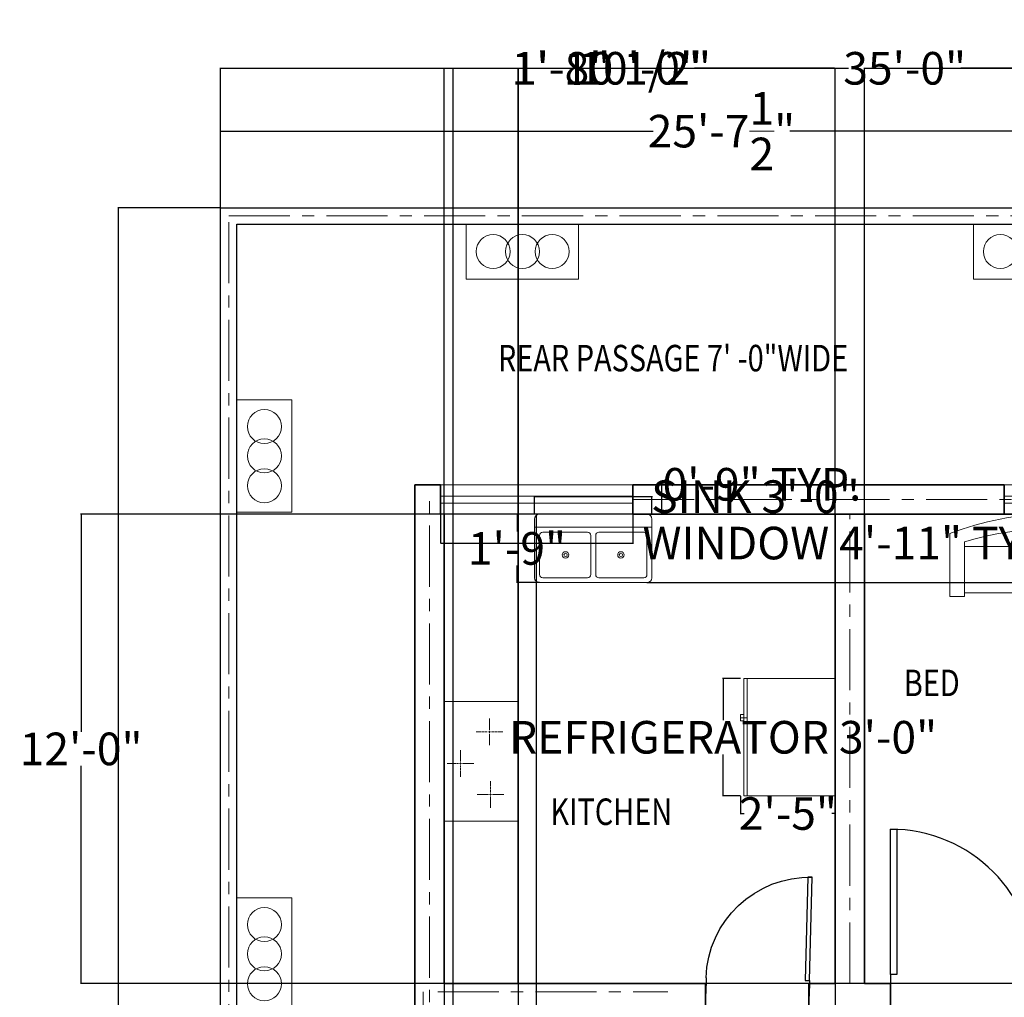
# Model space of a CAD drawing. Units: inches. Extents: x 541 to 1172, y -20 to 887.
# Tile 4 of 8: x 555 to 857, y 587 to 887. Entities that reach past the tile are written whole.
import ezdxf

# ---------------------------------------------------------------- set-up
doc = ezdxf.new("R2010")
doc.units = ezdxf.units.IN
doc.header["$MEASUREMENT"] = 0
doc.linetypes.add('CENTER', pattern=[50.8, 31.75, -6.35, 6.35, -6.35])
doc.linetypes.add('CENTER2', pattern=[1.125, 0.75, -0.125, 0.125, -0.125])
doc.layers.get('0').update_dxf_attribs({"color": 70})
for name, color, linetype, lineweight in [('A-ANNO-DIMS', 2, 'Continuous', 18), ('A-AREA-IDEN', 7, 'Continuous', 20), ('A-DOOR', 4, 'Continuous', 25), ('A-EQPM', 30, 'Continuous', 18), ('A-EQPM-CNTR', 30, 'CENTER2', 13), ('A-FLOR-CASE', 30, 'Continuous', 25), ('A-FLOR-FIXT', 9, 'Continuous', 18), ('A-FURN', 30, 'Continuous', 18), ('A-WALL-CNTR', 1, 'CENTER', 13), ('C-PROP', 7, 'Continuous', 25), ('L-PLNT', 70, 'Continuous', 18), ('L-SITE-WALL', 7, 'Continuous', 30), ('WALL', 7, 'Continuous', 35), ('WINDOW', 2, 'Continuous', 18)]:
    doc.layers.add(name, color=color, linetype=linetype, lineweight=lineweight)
doc.styles.get("Standard").update_dxf_attribs({"font": 'arial.ttf'})
doc.styles.add('YQ_DIM', font='SUPEROS.SHX', dxfattribs={"width": 0.8, "bigfont": 'HZDX.SHX'})
doc.dimstyles.get("Standard").update_dxf_attribs({"dimtxt": 10, "dimasz": 0.18, "dimexe": 0.18, "dimexo": 0.0625, "dimgap": 0.09, "dimtad": 0, "dimtih": 1, "dimtoh": 1, "dimdec": 1, "dimzin": 0, "dimdsep": 46, "dimlunit": 4, "dimtxsty": 'Standard', "dimcen": 0.09, "dimadec": 0, "dimazin": 0, "dimtfac": 1, "dimtdec": 1, "dimtofl": 0, "dimtmove": 0, "dimatfit": 3, "dimfxl": 1, "dimtolj": 1, "dimtzin": 0, "dimarcsym": 0})

# ---------------------------------------------------------------- blocks, each defined once
blk = doc.blocks.new('*D1')
at = {"layer": 'A-ANNO-DIMS', "color": 0, "lineweight": -2, "transparency": 16777216}
for p, q in [((616.64, 829.74), (616.64, 853.38)), ((616.82, 853.2), (749.39, 853.2)), ((923.96, 853.2), (791.38, 853.2)), ((924.14, 829.74), (924.14, 853.38))]:
    blk.add_line(p, q, dxfattribs=at)
for points in [[(616.82, 853.23), (616.82, 853.17), (616.64, 853.2)], [(923.96, 853.23), (923.96, 853.17), (924.14, 853.2)]]:
    blk.add_solid(points, dxfattribs=at)
at = {"layer": 'Defpoints', "color": 0, "lineweight": -2, "transparency": 16777216}
for p in [(616.64, 853.2), (616.64, 829.68), (924.14, 829.68)]:
    blk.add_point(p, dxfattribs=at)
at = {"layer": 'A-ANNO-DIMS', "color": 0, "transparency": 16777216, "insert": (770.39, 853.2), "char_height": 10, "attachment_point": 5}
blk.add_mtext('\\A1;25\'-7{\\H1x;\\S1/2;}"', dxfattribs=at)
blk = doc.blocks.new('*D3')
at = {"layer": 'A-ANNO-DIMS', "color": 0, "lineweight": -2, "transparency": 16777216}
for p, q in [((616.57, 829.68), (585.07, 829.68)), ((585.25, 829.5), (585.25, 539.38)), ((585.25, 238.86), (585.25, 528.98)), ((621.57, 238.68), (585.07, 238.68))]:
    blk.add_line(p, q, dxfattribs=at)
for points in [[(585.22, 829.5), (585.28, 829.5), (585.25, 829.68)], [(585.22, 238.86), (585.28, 238.86), (585.25, 238.68)]]:
    blk.add_solid(points, dxfattribs=at)
at = {"layer": 'Defpoints', "color": 0, "lineweight": -2, "transparency": 16777216}
for p in [(616.64, 829.68), (585.25, 238.68), (621.64, 238.68)]:
    blk.add_point(p, dxfattribs=at)
at = {"layer": 'A-ANNO-DIMS', "color": 0, "transparency": 16777216, "insert": (585.25, 534.18), "char_height": 10, "attachment_point": 5}
blk.add_mtext('\\A1;49\'-3"', dxfattribs=at)
blk = doc.blocks.new('Sofa - Roundback 7 ft.')
for p, q in [((-12.00002, -32.4421), (-12.00003, -6.5971)), ((11.99997, -32.4421), (11.99998, -6.5971)), ((-36.000027, -34), (-36.000027, -11.4696)), ((35.99998, -34), (35.99998, -11.4696)), ((-35.999844, -13.3819), (35.9998, -13.3819)), ((-36.000027, -32.4421), (35.99998, -32.4421))]:
    blk.add_line(p, q)
for points in [[(-36.000027, -34), (-42.000027, -34), (-42.000027, -8)], [(41.99998, -8), (41.99998, -34), (35.99998, -34)]]:
    blk.add_lwpolyline(points)
for centre, radius, start, end in [((0, -114.25), 114.25, 68.43141, 111.5686), ((-0.00001, -127.1968), 121.1968, 72.72033, 107.2797)]:
    blk.add_arc(centre, radius, start, end)
blk = doc.blocks.new('Refrigerator-2 door - 36 in top')
for p, q in [((0, -26.999999), (36, -26.999999)), ((12, -26.999999), (12, -28.999999)), ((11, -27.999999), (11, -28.999999)), ((11, -28.999999), (13, -28.999999)), ((13, -28.999999), (13, -27.999999))]:
    blk.add_line(p, q)
blk.add_lwpolyline([(0, -27.999999), (0, 0), (36, 0), (36, -27.999999)], close=True)
blk = doc.blocks.new('Sink-double - 36 in top')
for p, q in [((-18, -4), (18, -4)), ((-0.75, -18.5), (-0.75, -6.5)), ((0.75, -6.5), (0.75, -18.5))]:
    blk.add_line(p, q)
for points in [[(-16.5, 0), (16.5, 0)], [(-18, -19.5), (-18, -1.5)], [(18, -1.5), (18, -19.5)], [(-15.5, -5.5), (-1.75, -5.5)], [(1.75, -5.5), (15.5, -5.5)], [(-16.5, -18.5), (-16.5, -6.5)], [(16.5, -6.5), (16.5, -18.5)], [(16.5, -21), (-16.5, -21)], [(-1.75, -19.5), (-15.5, -19.5)], [(15.5, -19.5), (1.75, -19.5)]]:
    blk.add_lwpolyline(points)
for centre, radius in [((-8.5, -12.5), 1), ((-8.5, -12.5), 0.5), ((8.5, -12.5), 1), ((8.5, -12.5), 0.5)]:
    blk.add_circle(centre, radius)
for centre, radius, start, end in [((-16.5, -1.5), 1.5, 90, 180), ((16.5, -1.5), 1.5, 0, 90), ((-15.5, -6.5), 1, 90, 180), ((-1.75, -6.5), 1, 0, 90), ((1.75, -6.5), 1, 90, 180), ((15.5, -6.5), 1, 0, 90), ((-16.5, -19.5), 1.5, 180, 270), ((-15.5, -18.5), 1, 180, 270), ((-1.75, -18.5), 1, 270, 0), ((1.75, -18.5), 1, 180, 270), ((15.5, -18.5), 1, 270, 0), ((16.5, -19.5), 1.5, 270, 0)]:
    blk.add_arc(centre, radius, start, end)
blk = doc.blocks.new('*U19')
at = {"layer": 'A-EQPM-CNTR', "color": 0, "transparency": 16777216}
for p, q in [((0, 0.64), (0, 3.34)), ((-3.34, 0), (-0.64, 0)), ((0.64, 0), (3.34, 0)), ((0, -3.34), (0, -0.64))]:
    blk.add_line(p, q, dxfattribs=at)
at = {"layer": 'A-EQPM-CNTR', "color": 0, "linetype": 'Continuous', "transparency": 16777216}
for p, q in [((-0.32, 0), (0.32, 0)), ((0, -0.32), (0, 0.32))]:
    blk.add_line(p, q, dxfattribs=at)
blk = doc.blocks.new('*U20')
at = {"layer": 'A-EQPM-CNTR', "color": 0, "transparency": 16777216}
for p, q in [((0, 0.64), (0, 3.34)), ((-3.34, 0), (-0.64, 0)), ((0.64, 0), (3.34, 0)), ((0, -3.34), (0, -0.64))]:
    blk.add_line(p, q, dxfattribs=at)
at = {"layer": 'A-EQPM-CNTR', "color": 0, "linetype": 'Continuous', "transparency": 16777216}
for p, q in [((-0.32, 0), (0.32, 0)), ((0, -0.32), (0, 0.32))]:
    blk.add_line(p, q, dxfattribs=at)
blk = doc.blocks.new('*U21')
at = {"layer": 'A-EQPM-CNTR', "color": 0, "transparency": 16777216}
for p, q in [((0, 0.64), (0, 3.34)), ((-3.34, 0), (-0.64, 0)), ((0.64, 0), (3.34, 0)), ((0, -3.34), (0, -0.64))]:
    blk.add_line(p, q, dxfattribs=at)
at = {"layer": 'A-EQPM-CNTR', "color": 0, "linetype": 'Continuous', "transparency": 16777216}
for p, q in [((-0.32, 0), (0.32, 0)), ((0, -0.32), (0, 0.32))]:
    blk.add_line(p, q, dxfattribs=at)
blk = doc.blocks.new('*U23')
for p, q in [((0, 0), (0, -6)), ((40, 0), (40, -6))]:
    blk.add_line(p, q)
blk.add_lwpolyline([(0, 0), (0, 40), (1.75, 40), (1.75, 0)], close=True)
blk.add_arc((0, 0), 40, 0, 90)
blk = doc.blocks.new('WD_WIN4')
at = {"lineweight": -2}
for p, q in [((-0.5, 0.5), (0.5, 0.5)), ((-0.5, 0.12), (0.5, 0.12)), ((-0.5, -0.12), (0.5, -0.12)), ((-0.5, -0.5), (0.5, -0.5))]:
    blk.add_line(p, q, dxfattribs=at)
blk = doc.blocks.new('PLANTER-THREE-ROUND')
blk.add_lwpolyline([(34.49, 16.89), (0, 16.89), (0, 0), (34.49, 0)], close=True)
for centre in [(8.25, 8.45), (17.25, 8.45), (26.39, 8.45)]:
    blk.add_circle(centre, 5.21)
blk = doc.blocks.new('*D39')
at = {"layer": 'A-ANNO-DIMS', "color": 0, "lineweight": -2, "transparency": 16777216}
for p, q in [((684.16, 735.59), (684.16, 726.62)), ((743.21, 735.59), (743.21, 726.62)), ((684.34, 726.8), (743.03, 726.8)), ((743.21, 726.8), (743.39, 726.8))]:
    blk.add_line(p, q, dxfattribs=at)
for points in [[(684.34, 726.83), (684.34, 726.77), (684.16, 726.8)], [(743.03, 726.83), (743.03, 726.77), (743.21, 726.8)]]:
    blk.add_solid(points, dxfattribs=at)
at = {"layer": 'Defpoints', "color": 0, "lineweight": -2, "transparency": 16777216}
for p in [(684.16, 735.65), (743.21, 735.65), (743.21, 726.8)]:
    blk.add_point(p, dxfattribs=at)
at = {"layer": 'A-ANNO-DIMS', "color": 0, "transparency": 16777216, "insert": (810.64, 726.8), "char_height": 10, "attachment_point": 5}
blk.add_mtext('\\A1;WINDOW 4\'-11" TYP.', dxfattribs=at)
blk = doc.blocks.new('*D40')
at = {"layer": 'A-ANNO-DIMS', "color": 0, "lineweight": -2, "transparency": 16777216}
for p, q in [((743.27, 744.65), (752.25, 744.65)), ((752.07, 744.65), (752.07, 744.83)), ((752.07, 744.83), (752.25, 744.83)), ((752.07, 735.83), (752.07, 744.47)), ((743.27, 735.65), (752.25, 735.65))]:
    blk.add_line(p, q, dxfattribs=at)
for points in [[(752.04, 744.47), (752.1, 744.47), (752.07, 744.65)], [(752.04, 735.83), (752.1, 735.83), (752.07, 735.65)]]:
    blk.add_solid(points, dxfattribs=at)
at = {"layer": 'Defpoints', "color": 0, "lineweight": -2, "transparency": 16777216}
for p in [(743.21, 744.65), (752.07, 744.65), (743.21, 735.65)]:
    blk.add_point(p, dxfattribs=at)
at = {"layer": 'A-ANNO-DIMS', "color": 0, "transparency": 16777216, "insert": (782.82, 744.83), "char_height": 10, "attachment_point": 5}
blk.add_mtext('\\A1;0\'-9" TYP.', dxfattribs=at)
blk = doc.blocks.new('*D49')
at = {"layer": 'A-ANNO-DIMS', "color": 0, "lineweight": -2, "transparency": 16777216}
for p, q in [((713.03, 735.72), (713.03, 741.23)), ((713.21, 741.05), (748.85, 741.05)), ((749.03, 735.72), (749.03, 741.23)), ((749.03, 741.05), (749.21, 741.05))]:
    blk.add_line(p, q, dxfattribs=at)
for points in [[(713.21, 741.08), (713.21, 741.02), (713.03, 741.05)], [(748.85, 741.08), (748.85, 741.02), (749.03, 741.05)]]:
    blk.add_solid(points, dxfattribs=at)
at = {"layer": 'Defpoints', "color": 0, "lineweight": -2, "transparency": 16777216}
for p in [(749.03, 741.05), (713.03, 735.65), (749.03, 735.65)]:
    blk.add_point(p, dxfattribs=at)
at = {"layer": 'A-ANNO-DIMS', "color": 0, "transparency": 16777216, "insert": (780.81, 741.05), "char_height": 10, "attachment_point": 5}
blk.add_mtext('\\A1;SINK 3\'-0"', dxfattribs=at)
blk = doc.blocks.new('*D50')
at = {"layer": 'A-ANNO-DIMS', "color": 0, "lineweight": -2, "transparency": 16777216}
for p, q in [((712.97, 735.65), (707.45, 735.65)), ((707.63, 735.47), (707.63, 730.35)), ((707.63, 714.83), (707.63, 719.96)), ((712.97, 714.65), (707.45, 714.65))]:
    blk.add_line(p, q, dxfattribs=at)
for points in [[(707.6, 735.47), (707.66, 735.47), (707.63, 735.65)], [(707.6, 714.83), (707.66, 714.83), (707.63, 714.65)]]:
    blk.add_solid(points, dxfattribs=at)
at = {"layer": 'Defpoints', "color": 0, "lineweight": -2, "transparency": 16777216}
for p in [(707.63, 735.65), (713.03, 735.65), (713.03, 714.65)]:
    blk.add_point(p, dxfattribs=at)
at = {"layer": 'A-ANNO-DIMS', "color": 0, "transparency": 16777216, "insert": (707.63, 725.15), "char_height": 10, "attachment_point": 5}
blk.add_mtext('\\A1;1\'-9"', dxfattribs=at)
blk = doc.blocks.new('*D61')
at = {"layer": 'A-ANNO-DIMS', "color": 0, "lineweight": -2, "transparency": 16777216}
for p, q in [((802.49, 574.25), (802.49, 579.28)), ((802.67, 579.1), (835.09, 579.1)), ((835.27, 574.25), (835.27, 579.28)), ((835.27, 579.1), (835.45, 579.1))]:
    blk.add_line(p, q, dxfattribs=at)
for points in [[(802.67, 579.13), (802.67, 579.07), (802.49, 579.1)], [(835.09, 579.13), (835.09, 579.07), (835.27, 579.1)]]:
    blk.add_solid(points, dxfattribs=at)
at = {"layer": 'Defpoints', "color": 0, "lineweight": -2, "transparency": 16777216}
for p in [(835.27, 579.1), (802.49, 574.19), (835.27, 574.19)]:
    blk.add_point(p, dxfattribs=at)
at = {"layer": 'A-ANNO-DIMS', "color": 0, "transparency": 16777216, "insert": (896.96, 579.1), "char_height": 10, "attachment_point": 5}
blk.add_mtext('\\A1;ACCENT 2\'-9" TYP.', dxfattribs=at)
blk = doc.blocks.new('*D65')
at = {"layer": 'A-ANNO-DIMS', "color": 0, "lineweight": -2, "transparency": 16777216}
for p, q in [((776.22, 685.21), (770.7, 685.21)), ((770.88, 685.03), (770.88, 672.48)), ((770.88, 649.39), (770.88, 661.94)), ((776.22, 649.21), (770.7, 649.21))]:
    blk.add_line(p, q, dxfattribs=at)
for points in [[(770.85, 685.03), (770.91, 685.03), (770.88, 685.21)], [(770.85, 649.39), (770.91, 649.39), (770.88, 649.21)]]:
    blk.add_solid(points, dxfattribs=at)
at = {"layer": 'Defpoints', "color": 0, "lineweight": -2, "transparency": 16777216}
for p in [(776.28, 685.21), (770.88, 649.21), (776.28, 649.21)]:
    blk.add_point(p, dxfattribs=at)
at = {"layer": 'A-ANNO-DIMS', "color": 0, "transparency": 16777216, "insert": (770.88, 667.21), "char_height": 10, "attachment_point": 5}
blk.add_mtext('\\A1;REFRIGERATOR 3\'-0"', dxfattribs=at)
blk = doc.blocks.new('*D66')
at = {"layer": 'A-ANNO-DIMS', "color": 0, "lineweight": -2, "transparency": 16777216}
for p, q in [((776.28, 649.15), (776.28, 643.63)), ((805.28, 649.15), (805.28, 643.63)), ((776.46, 643.81), (777.32, 643.81)), ((805.1, 643.81), (804.25, 643.81))]:
    blk.add_line(p, q, dxfattribs=at)
for points in [[(776.46, 643.84), (776.46, 643.78), (776.28, 643.81)], [(805.1, 643.84), (805.1, 643.78), (805.28, 643.81)]]:
    blk.add_solid(points, dxfattribs=at)
at = {"layer": 'Defpoints', "color": 0, "lineweight": -2, "transparency": 16777216}
for p in [(776.28, 649.21), (805.28, 649.21), (805.28, 643.81)]:
    blk.add_point(p, dxfattribs=at)
at = {"layer": 'A-ANNO-DIMS', "color": 0, "transparency": 16777216, "insert": (790.78, 643.81), "char_height": 10, "attachment_point": 5}
blk.add_mtext('\\A1;2\'-5"', dxfattribs=at)
blk = doc.blocks.new('*D69')
at = {"layer": 'A-ANNO-DIMS', "color": 0, "lineweight": -2, "transparency": 16777216}
for p, q in [((616.64, 829.74), (616.64, 872.66)), ((616.82, 872.48), (809.37, 872.48)), ((1036.46, 872.48), (843.9, 872.48)), ((1036.64, 829.74), (1036.64, 872.66))]:
    blk.add_line(p, q, dxfattribs=at)
for points in [[(616.82, 872.51), (616.82, 872.45), (616.64, 872.48)], [(1036.46, 872.51), (1036.46, 872.45), (1036.64, 872.48)]]:
    blk.add_solid(points, dxfattribs=at)
at = {"layer": 'Defpoints', "color": 0, "lineweight": -2, "transparency": 16777216}
for p in [(1036.64, 872.48), (616.64, 829.68), (1036.64, 829.68)]:
    blk.add_point(p, dxfattribs=at)
at = {"layer": 'A-ANNO-DIMS', "color": 0, "transparency": 16777216, "insert": (826.64, 872.48), "char_height": 10, "attachment_point": 5}
blk.add_mtext('\\A1;35\'-0"', dxfattribs=at)
blk = doc.blocks.new('*D75')
at = {"layer": 'A-ANNO-DIMS', "color": 0, "lineweight": -2, "transparency": 16777216}
for p, q in [((685.28, 735.72), (685.28, 872.66)), ((685.46, 872.48), (728.49, 872.48)), ((805.1, 872.48), (762.08, 872.48)), ((805.28, 735.72), (805.28, 872.66))]:
    blk.add_line(p, q, dxfattribs=at)
for points in [[(685.46, 872.51), (685.46, 872.45), (685.28, 872.48)], [(805.1, 872.51), (805.1, 872.45), (805.28, 872.48)]]:
    blk.add_solid(points, dxfattribs=at)
at = {"layer": 'Defpoints', "color": 0, "lineweight": -2, "transparency": 16777216}
for p in [(805.28, 872.48), (685.28, 735.65), (805.28, 735.65)]:
    blk.add_point(p, dxfattribs=at)
at = {"layer": 'A-ANNO-DIMS', "color": 0, "transparency": 16777216, "insert": (745.28, 872.48), "char_height": 10, "attachment_point": 5}
blk.add_mtext('\\A1;10\'-0"', dxfattribs=at)
blk = doc.blocks.new('*D76')
at = {"layer": 'A-ANNO-DIMS', "color": 0, "lineweight": -2, "transparency": 16777216}
for p, q in [((814.28, 735.72), (814.28, 872.66)), ((814.46, 872.48), (873.99, 872.48)), ((967.1, 872.48), (907.58, 872.48)), ((967.28, 735.72), (967.28, 872.66))]:
    blk.add_line(p, q, dxfattribs=at)
for points in [[(814.46, 872.51), (814.46, 872.45), (814.28, 872.48)], [(967.1, 872.51), (967.1, 872.45), (967.28, 872.48)]]:
    blk.add_solid(points, dxfattribs=at)
at = {"layer": 'Defpoints', "color": 0, "lineweight": -2, "transparency": 16777216}
for p in [(967.28, 872.48), (814.28, 735.65), (967.28, 735.65)]:
    blk.add_point(p, dxfattribs=at)
at = {"layer": 'A-ANNO-DIMS', "color": 0, "transparency": 16777216, "insert": (890.78, 872.48), "char_height": 10, "attachment_point": 5}
blk.add_mtext('\\A1;12\'-9"', dxfattribs=at)
blk = doc.blocks.new('*D78')
at = {"layer": 'A-ANNO-DIMS', "color": 0, "lineweight": -2, "transparency": 16777216}
for p, q in [((685.22, 735.65), (573.66, 735.65)), ((573.84, 735.47), (573.84, 668.85)), ((573.84, 591.83), (573.84, 658.46)), ((685.22, 591.65), (573.66, 591.65))]:
    blk.add_line(p, q, dxfattribs=at)
for points in [[(573.81, 735.47), (573.87, 735.47), (573.84, 735.65)], [(573.81, 591.83), (573.87, 591.83), (573.84, 591.65)]]:
    blk.add_solid(points, dxfattribs=at)
at = {"layer": 'Defpoints', "color": 0, "lineweight": -2, "transparency": 16777216}
for p in [(685.28, 735.65), (573.84, 591.65), (685.28, 591.65)]:
    blk.add_point(p, dxfattribs=at)
at = {"layer": 'A-ANNO-DIMS', "color": 0, "transparency": 16777216, "insert": (573.84, 663.65), "char_height": 10, "attachment_point": 5}
blk.add_mtext('\\A1;12\'-0"', dxfattribs=at)
blk = doc.blocks.new('*D99')
at = {"layer": 'A-ANNO-DIMS', "color": 0, "lineweight": -2, "transparency": 16777216}
for p, q in [((765.53, 591.59), (765.53, -5.37)), ((797.19, 591.59), (797.19, -5.37)), ((765.71, -5.19), (797.01, -5.19)), ((797.19, -5.19), (797.37, -5.19))]:
    blk.add_line(p, q, dxfattribs=at)
for points in [[(765.71, -5.16), (765.71, -5.22), (765.53, -5.19)], [(797.01, -5.16), (797.01, -5.22), (797.19, -5.19)]]:
    blk.add_solid(points, dxfattribs=at)
at = {"layer": 'Defpoints', "color": 0, "lineweight": -2, "transparency": 16777216}
for p in [(765.53, 591.65), (797.19, 591.65), (797.19, -5.19)]:
    blk.add_point(p, dxfattribs=at)
at = {"layer": 'A-ANNO-DIMS', "color": 0, "transparency": 16777216, "insert": (822.49, -5.19), "char_height": 10, "attachment_point": 5}
blk.add_mtext('\\A1;2\'-7 1/2"', dxfattribs=at)
blk = doc.blocks.new('*D100')
at = {"layer": 'A-ANNO-DIMS', "color": 0, "lineweight": -2, "transparency": 16777216}
for p, q in [((685.28, 591.72), (685.28, 872.66)), ((685.46, 872.48), (707.76, 872.48)), ((707.94, 591.72), (707.94, 872.66)), ((707.94, 872.48), (708.12, 872.48))]:
    blk.add_line(p, q, dxfattribs=at)
for points in [[(685.46, 872.51), (685.46, 872.45), (685.28, 872.48)], [(707.76, 872.51), (707.76, 872.45), (707.94, 872.48)]]:
    blk.add_solid(points, dxfattribs=at)
at = {"layer": 'Defpoints', "color": 0, "lineweight": -2, "transparency": 16777216}
for p in [(707.94, 872.48), (685.28, 591.65), (707.94, 591.65)]:
    blk.add_point(p, dxfattribs=at)
at = {"layer": 'A-ANNO-DIMS', "color": 0, "transparency": 16777216, "insert": (736.56, 872.48), "char_height": 10, "attachment_point": 5}
blk.add_mtext('\\A1;1\'-10 1/2"', dxfattribs=at)
blk = doc.blocks.new('*D101')
at = {"layer": 'A-ANNO-DIMS', "color": 0, "lineweight": -2, "transparency": 16777216}
for p, q in [((805.35, 735.65), (1143.21, 735.65)), ((1143.03, 735.47), (1143.03, 730.35)), ((1143.03, 714.83), (1143.03, 719.96)), ((805.35, 714.65), (1143.21, 714.65))]:
    blk.add_line(p, q, dxfattribs=at)
for points in [[(1143, 735.47), (1143.06, 735.47), (1143.03, 735.65)], [(1143, 714.83), (1143.06, 714.83), (1143.03, 714.65)]]:
    blk.add_solid(points, dxfattribs=at)
at = {"layer": 'Defpoints', "color": 0, "lineweight": -2, "transparency": 16777216}
for p in [(805.28, 735.65), (1143.03, 735.65), (805.28, 714.65)]:
    blk.add_point(p, dxfattribs=at)
at = {"layer": 'A-ANNO-DIMS', "color": 0, "transparency": 16777216, "insert": (1143.03, 725.15), "char_height": 10, "attachment_point": 5}
blk.add_mtext('\\A1;1\'-9"', dxfattribs=at)
blk = doc.blocks.new('*D105')
at = {"layer": 'A-ANNO-DIMS', "color": 0, "lineweight": -2, "transparency": 16777216}
for p, q in [((797.19, 591.59), (797.19, -5.37)), ((805.28, 591.59), (805.28, -5.37)), ((797.37, -5.19), (805.1, -5.19)), ((805.28, -5.19), (805.46, -5.19))]:
    blk.add_line(p, q, dxfattribs=at)
for points in [[(797.37, -5.16), (797.37, -5.22), (797.19, -5.19)], [(805.1, -5.16), (805.1, -5.22), (805.28, -5.19)]]:
    blk.add_solid(points, dxfattribs=at)
at = {"layer": 'Defpoints', "color": 0, "lineweight": -2, "transparency": 16777216}
for p in [(797.19, 591.65), (805.28, 591.65), (805.28, -5.19)]:
    blk.add_point(p, dxfattribs=at)
at = {"layer": 'A-ANNO-DIMS', "color": 0, "transparency": 16777216, "insert": (818.84, -5.19), "char_height": 10, "attachment_point": 5}
blk.add_mtext('\\A1;0\'-8"', dxfattribs=at)
blk = doc.blocks.new('*D106')
at = {"layer": 'A-ANNO-DIMS', "color": 0, "lineweight": -2, "transparency": 16777216}
for p, q in [((685.28, 735.59), (685.28, -5.37)), ((713.47, 735.15), (713.47, -5.37)), ((685.46, -5.19), (685.91, -5.19)), ((713.29, -5.19), (712.84, -5.19))]:
    blk.add_line(p, q, dxfattribs=at)
for points in [[(685.46, -5.16), (685.46, -5.22), (685.28, -5.19)], [(713.29, -5.16), (713.29, -5.22), (713.47, -5.19)]]:
    blk.add_solid(points, dxfattribs=at)
at = {"layer": 'Defpoints', "color": 0, "lineweight": -2, "transparency": 16777216}
for p in [(685.28, 735.65), (713.47, 735.22), (685.28, -5.19)]:
    blk.add_point(p, dxfattribs=at)
at = {"layer": 'A-ANNO-DIMS', "color": 0, "transparency": 16777216, "insert": (699.38, -5.19), "char_height": 10, "attachment_point": 5}
blk.add_mtext('\\A1;2\'-4"', dxfattribs=at)
blk = doc.blocks.new('*D107')
at = {"layer": 'A-ANNO-DIMS', "color": 0, "lineweight": -2, "transparency": 16777216}
for p, q in [((967.22, 735.65), (573.66, 735.65)), ((573.84, 735.47), (573.84, 668.85)), ((573.84, 591.83), (573.84, 658.46)), ((967.22, 591.65), (573.66, 591.65))]:
    blk.add_line(p, q, dxfattribs=at)
for points in [[(573.81, 735.47), (573.87, 735.47), (573.84, 735.65)], [(573.81, 591.83), (573.87, 591.83), (573.84, 591.65)]]:
    blk.add_solid(points, dxfattribs=at)
at = {"layer": 'Defpoints', "color": 0, "lineweight": -2, "transparency": 16777216}
for p in [(967.28, 735.65), (573.84, 591.65), (967.28, 591.65)]:
    blk.add_point(p, dxfattribs=at)
at = {"layer": 'A-ANNO-DIMS', "color": 0, "transparency": 16777216, "insert": (573.84, 663.65), "char_height": 10, "attachment_point": 5}
blk.add_mtext('\\A1;12\'-0"', dxfattribs=at)
blk = doc.blocks.new('*D110')
at = {"layer": 'A-ANNO-DIMS', "color": 0, "lineweight": -2, "transparency": 16777216}
for p, q in [((688.04, 521.72), (688.04, 872.66)), ((688.22, 872.48), (707.94, 872.48)), ((708.12, 521.72), (708.12, 872.66)), ((708.12, 872.48), (708.3, 872.48))]:
    blk.add_line(p, q, dxfattribs=at)
for points in [[(688.22, 872.51), (688.22, 872.45), (688.04, 872.48)], [(707.94, 872.51), (707.94, 872.45), (708.12, 872.48)]]:
    blk.add_solid(points, dxfattribs=at)
at = {"layer": 'Defpoints', "color": 0, "lineweight": -2, "transparency": 16777216}
for p in [(708.12, 872.48), (688.04, 521.65), (708.12, 521.65)]:
    blk.add_point(p, dxfattribs=at)
at = {"layer": 'A-ANNO-DIMS', "color": 0, "transparency": 16777216, "insert": (721.21, 872.48), "char_height": 10, "attachment_point": 5}
blk.add_mtext('\\A1;1\'-8"', dxfattribs=at)

msp = doc.modelspace()

# ---------------------------------------------------------------- linework, layer by layer
at = {"layer": 'A-EQPM'}
for p, q in [((685.28, 678.22), (707.94, 678.22)), ((699.16, 672.99), (699.16, 672.23)), ((695.82, 668.88), (695.05, 668.88)), ((702.51, 668.88), (703.27, 668.88)), ((699.16, 664.78), (699.16, 665.54)), ((690.31, 663.28), (690.31, 662.52)), ((686.97, 659.18), (686.2, 659.18)), ((693.65, 659.18), (694.42, 659.18)), ((690.31, 655.07), (690.31, 655.83)), ((699.5, 653.75), (699.5, 652.99)), ((696.16, 649.64), (695.39, 649.64)), ((702.84, 649.64), (703.61, 649.64)), ((699.5, 645.54), (699.5, 646.3)), ((707.94, 641.43), (685.28, 641.43))]:
    msp.add_line(p, q, dxfattribs=at)
at = {"layer": 'A-FLOR-CASE'}
for p, q in [((714.53, 714.65), (707.94, 714.65)), ((707.94, 714.65), (707.94, 591.65)), ((747.53, 714.65), (805.28, 714.65))]:
    msp.add_line(p, q, dxfattribs=at)
at = {"layer": 'A-WALL-CNTR', "ltscale": 0.590551}
for p, q in [((619.14, 827.18), (1034.15, 827.18)), ((619.14, 56.56), (619.14, 827.18)), ((680.78, 233.42), (680.78, 740.15)), ((743.21, 740.15), (926.64, 740.15)), ((809.78, 591.65), (809.78, 735.65)), ((678.78, 524.15), (678.78, 589.15)), ((683.28, 589.15), (753.91, 589.15))]:
    msp.add_line(p, q, dxfattribs=at)
at = {"layer": 'C-PROP'}
msp.add_line((616.64, 829.68), (1036.64, 829.68), dxfattribs=at)
at = {"layer": 'L-SITE-WALL'}
for p, q in [((616.64, 49.68), (616.64, 829.68)), ((616.64, 829.68), (1036.64, 829.68)), ((621.64, 238.68), (621.64, 824.68)), ((621.64, 824.68), (924.14, 824.68))]:
    msp.add_line(p, q, dxfattribs=at)
at = {"layer": 'WALL'}
for p, q in [((676.28, 744.65), (684.16, 744.65)), ((676.28, 439.71), (676.28, 744.65)), ((684.16, 744.65), (684.16, 735.65)), ((743.21, 744.65), (857.21, 744.65)), ((743.21, 744.65), (743.21, 735.65)), ((857.21, 744.65), (857.21, 735.65)), ((685.28, 591.65), (685.28, 735.65)), ((743.21, 735.65), (805.28, 735.65)), ((805.28, 591.65), (805.28, 735.65)), ((814.28, 591.65), (814.28, 735.65)), ((814.28, 735.65), (857.21, 735.65)), ((685.28, 591.65), (765.53, 591.65)), ((765.53, 582.65), (765.53, 591.65)), ((797.19, 591.65), (797.19, 582.65)), ((797.19, 591.65), (805.28, 591.65)), ((814.28, 591.65), (822.26, 591.65)), ((822.26, 591.65), (822.26, 582.65))]:
    msp.add_line(p, q, dxfattribs=at)

# ---------------------------------------------------------------- block references
at = {"layer": 'A-DOOR', "xscale": 1.115231810502029, "yscale": 1.115231810502029, "zscale": 1.115231810502029}
msp.add_blockref('*U23', (822.26, 594.38), dxfattribs=at)
at = {"layer": 'A-DOOR', "xscale": -0.7934318724739616, "yscale": 0.7934318724739615, "zscale": 0.7934318724739615, "rotation": 358.4510988302025}
msp.add_blockref('*U23', (797.42, 592.53), dxfattribs=at)
at = {"layer": 'A-EQPM', "rotation": 270}
msp.add_blockref('Refrigerator-2 door - 36 in top', (805.28, 685.21), dxfattribs=at)
at = {"layer": 'A-EQPM-CNTR'}
for name, p in [('*U20', (699.16, 668.88)), ('*U19', (690.31, 659.18)), ('*U21', (699.5, 649.64))]:
    msp.add_blockref(name, p, dxfattribs=at)
at = {"layer": 'A-FLOR-FIXT'}
msp.add_blockref('Sink-double - 36 in top', (731.03, 735.65), dxfattribs=at)
at = {"layer": 'A-FURN', "xscale": 0.7424226432878923, "yscale": 0.7424226432878923, "zscale": 0.7424226432878923}
msp.add_blockref('Sofa - Roundback 7 ft.', (871.71, 735.65), dxfattribs=at)
at = {"layer": 'L-PLNT'}
for p in [(692.04, 807.79), (847.75, 807.79)]:
    msp.add_blockref('PLANTER-THREE-ROUND', p, dxfattribs=at)
for p, rotation in [((621.64, 770.79), 269.9999999999999), ((621.64, 617.98), 269.9999999999998)]:
    msp.add_blockref('PLANTER-THREE-ROUND', p, dxfattribs=dict(at, rotation=rotation))
at = {"layer": 'WINDOW', "xscale": 59.05511811023622, "zscale": 59.05511811023622}
for p, yscale, rotation in [((713.68, 740.15), 9.000000000000114, 359.9999999999999), ((886.73, 740.15), 9, 179.9999999999998)]:
    msp.add_blockref('WD_WIN4', p, dxfattribs=dict(at, yscale=yscale, rotation=rotation))

# ---------------------------------------------------------------- texts
at = {"layer": 'A-AREA-IDEN', "style": 'YQ_DIM', "width": 0.8}
for s, height, p in [('REAR PASSAGE 7\' -0"WIDE', 8.1299, (701.78, 779.48)), (' BED', 8.13, (824.37, 679.83)), (' KITCHEN', 8.13, (715.87, 640.3))]:
    msp.add_text(s, height=height, dxfattribs=at).set_placement(p)

# ---------------------------------------------------------------- dimensions: what is measured, and where the dimension line sits
at = {"layer": 'A-ANNO-DIMS'}
for base, p1, p2, override, picture, middle in [((707.94, 872.48), (685.28, 591.65), (707.94, 591.65), {"dimdec": 1, "dimlfac": 1, "dimrnd": 0, "dimzin": 1, "dimdsep": 46, "dimlunit": 4, "dimfrac": 2}, '*D100', (736.56, 872.48)), ((1036.64, 872.48), (616.64, 829.68), (1036.64, 829.68), {"dimdec": 1, "dimlfac": 1, "dimrnd": 0, "dimzin": 1, "dimdsep": 46, "dimlunit": 4, "dimfrac": 2}, '*D69', (826.64, 872.48)), ((805.28, 872.48), (685.28, 735.65), (805.28, 735.65), {"dimdec": 1, "dimlfac": 1, "dimrnd": 0, "dimzin": 1, "dimdsep": 46, "dimlunit": 4, "dimfrac": 2}, '*D75', (745.28, 872.48)), ((708.12, 872.48), (688.04, 521.65), (708.12, 521.65), {"dimdec": 1, "dimlfac": 1, "dimrnd": 0, "dimzin": 1, "dimdsep": 46, "dimlunit": 4, "dimfrac": 2}, '*D110', (721.21, 872.48)), ((967.28, 872.48), (814.28, 735.65), (967.28, 735.65), {"dimdec": 1, "dimlfac": 1, "dimrnd": 0, "dimzin": 1, "dimdsep": 46, "dimlunit": 4, "dimfrac": 2}, '*D76', (890.78, 872.48)), ((616.64, 853.2), (924.14, 829.68), (616.64, 829.68), {"dimclrd": 0, "dimclre": 0, "dimclrt": 0}, '*D1', (770.39, 853.2)), ((685.28, -5.19), (713.47, 735.22), (685.28, 735.65), {"dimdec": 1, "dimlfac": 1, "dimrnd": 0, "dimzin": 1, "dimdsep": 46, "dimlunit": 4, "dimfrac": 2}, '*D106', (699.38, -5.19)), ((805.28, 643.81), (776.28, 649.21), (805.28, 649.21), {"dimdec": 1, "dimlfac": 1, "dimrnd": 0, "dimzin": 1, "dimdsep": 46, "dimlunit": 4, "dimfrac": 2}, '*D66', (790.78, 643.81)), ((797.19, -5.19), (765.53, 591.65), (797.19, 591.65), {"dimdec": 1, "dimlfac": 1, "dimrnd": 0, "dimzin": 1, "dimdsep": 46, "dimlunit": 4, "dimfrac": 2}, '*D99', (822.49, -5.19)), ((805.28, -5.19), (797.19, 591.65), (805.28, 591.65), {"dimdec": 1, "dimlfac": 1, "dimrnd": 0, "dimzin": 1, "dimdsep": 46, "dimlunit": 4, "dimfrac": 2}, '*D105', (818.84, -5.19))]:
    dim = msp.add_linear_dim(base=base, p1=p1, p2=p2, dimstyle='Standard', override=override, dxfattribs=at)
    dim.commit()
    dim.dimension.update_dxf_attribs({"geometry": picture, "text_midpoint": middle})
for base, p1, p2, override, picture, middle in [((585.25, 238.68), (616.64, 829.68), (621.64, 238.68), {"dimclrd": 0, "dimclre": 0, "dimclrt": 0}, '*D3', (585.25, 534.18)), ((573.84, 591.65), (685.28, 735.65), (685.28, 591.65), {"dimdec": 1, "dimlfac": 1, "dimrnd": 0, "dimzin": 1, "dimdsep": 46, "dimlunit": 4, "dimfrac": 2}, '*D78', (573.84, 663.65)), ((573.84, 591.65), (967.28, 735.65), (967.28, 591.65), {"dimdec": 1, "dimlfac": 1, "dimrnd": 0, "dimzin": 1, "dimdsep": 46, "dimlunit": 4, "dimfrac": 2}, '*D107', (573.84, 663.65)), ((707.63, 735.65), (713.03, 714.65), (713.03, 735.65), {"dimdec": 1, "dimlfac": 1, "dimrnd": 0, "dimzin": 1, "dimdsep": 46, "dimlunit": 4, "dimfrac": 2}, '*D50', (707.63, 725.15)), ((1143.03, 735.65), (805.28, 714.65), (805.28, 735.65), {"dimdec": 1, "dimlfac": 1, "dimrnd": 0, "dimzin": 1, "dimdsep": 46, "dimlunit": 4, "dimfrac": 2}, '*D101', (1143.03, 725.15))]:
    dim = msp.add_linear_dim(base=base, p1=p1, p2=p2, angle=90, dimstyle='Standard', override=override, dxfattribs=at)
    dim.commit()
    dim.dimension.update_dxf_attribs({"geometry": picture, "text_midpoint": middle})
for base, p1, p2, angle, text, picture, middle in [((752.07, 744.65), (743.21, 735.65), (743.21, 744.65), 90, '<> TYP.', '*D40', (782.82, 744.83)), ((770.88, 649.21), (776.28, 685.21), (776.28, 649.21), 270, 'REFRIGERATOR <>', '*D65', (770.88, 667.21))]:
    dim = msp.add_linear_dim(base=base, p1=p1, p2=p2, angle=angle, text=text, dimstyle='Standard', override={"dimdec": 1, "dimlfac": 1, "dimrnd": 0, "dimzin": 1, "dimdsep": 46, "dimlunit": 4, "dimfrac": 2}, dxfattribs=at)
    dim.commit()
    dim.dimension.update_dxf_attribs({"geometry": picture, "text_midpoint": middle})
for base, p1, p2, text, picture, middle in [((749.03, 741.05), (713.03, 735.65), (749.03, 735.65), 'SINK <>', '*D49', (780.81, 741.05)), ((743.2125, 726.7962), (684.1574, 735.6544), (743.2125, 735.6544), 'WINDOW <> TYP.', '*D39', (810.638, 726.7962)), ((835.27, 579.1), (802.49, 574.19), (835.27, 574.19), 'ACCENT <> TYP.', '*D61', (896.96, 579.1))]:
    dim = msp.add_linear_dim(base=base, p1=p1, p2=p2, text=text, dimstyle='Standard', override={"dimdec": 1, "dimlfac": 1, "dimrnd": 0, "dimzin": 1, "dimdsep": 46, "dimlunit": 4, "dimfrac": 2}, dxfattribs=at)
    dim.commit()
    dim.dimension.update_dxf_attribs({"geometry": picture, "text_midpoint": middle})

doc.saveas('drawing.dxf')
